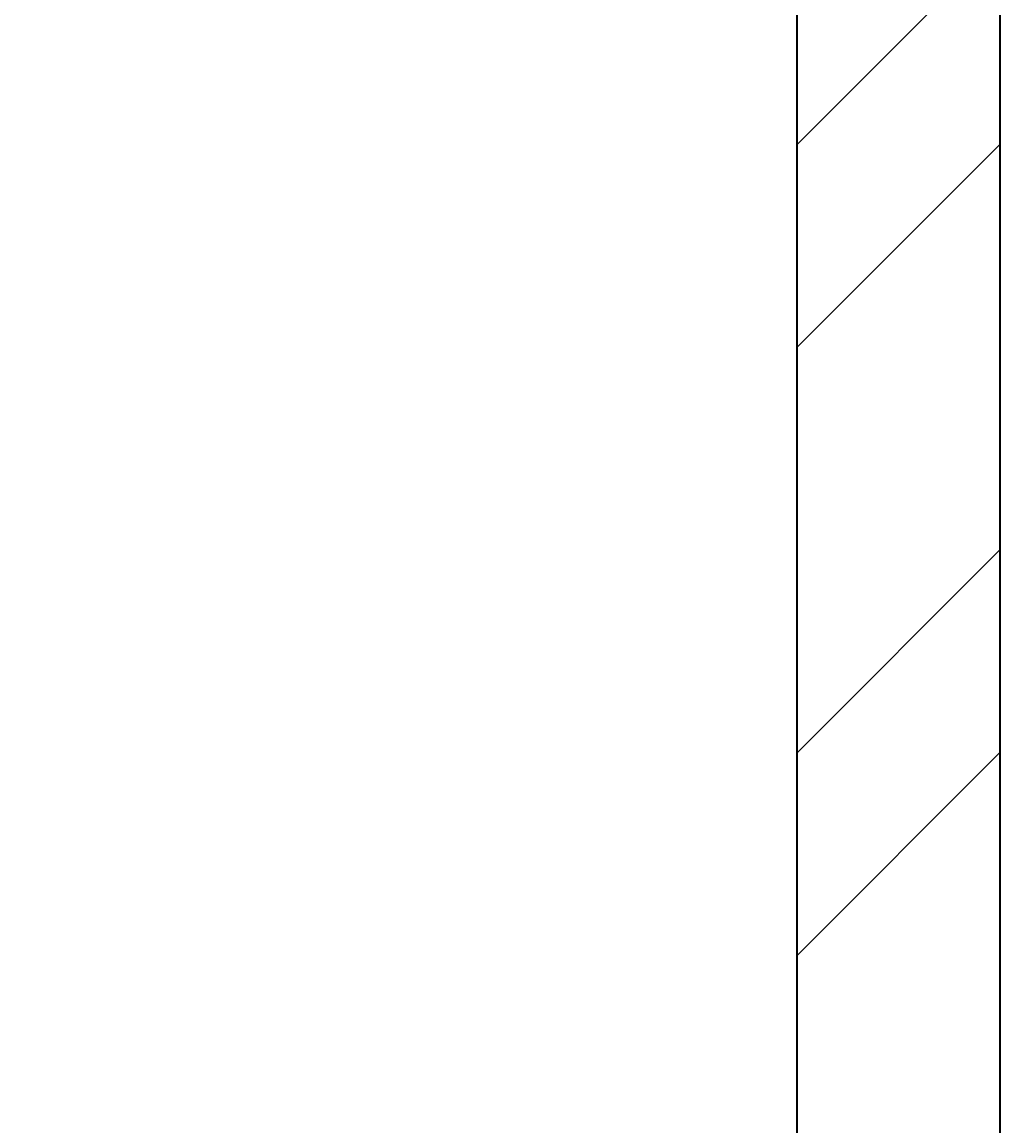
# Model space of a CAD drawing. Units: inches. Extents: x 1962 to 2771, y 1245 to 2660.
# Tile 79 of 114: x 2639 to 2661, y 2082 to 2107. Entities that reach past the tile are written whole.
import ezdxf

# ---------------------------------------------------------------- set-up
doc = ezdxf.new("R2010")
doc.units = ezdxf.units.IN
for name, color, linetype, lineweight in [('A-ANNO-DIMS', 2, 'Continuous', 18), ('A-WALL', 7, 'Continuous', 35), ('A-WALL-PATT', 252, 'Continuous', 13)]:
    doc.layers.add(name, color=color, linetype=linetype, lineweight=lineweight)
doc.styles.get("Standard").update_dxf_attribs({"font": 'arial.ttf'})
doc.dimstyles.get("Standard").update_dxf_attribs({"dimtxt": 0.18, "dimasz": 0.18, "dimexe": 0.18, "dimexo": 0.0625, "dimgap": 0.09, "dimtad": 0, "dimtih": 1, "dimtoh": 1, "dimdec": 4, "dimzin": 0, "dimdsep": 46, "dimtxsty": 'Standard', "dimcen": 0.09, "dimadec": 0, "dimazin": 0, "dimtfac": 1, "dimtdec": 4, "dimtofl": 0, "dimtmove": 0, "dimatfit": 3, "dimfxl": 1, "dimtolj": 1, "dimtzin": 0, "dimarcsym": 0})

# ---------------------------------------------------------------- blocks, each defined once
blk = doc.blocks.new('*D40')
at = {"layer": 'A-ANNO-DIMS', "color": 0, "lineweight": -2, "transparency": 16777216}
for p, q in [((2072.02, 2033.906), (2072.02, 2583.474)), ((2660.807, 2524.406), (2660.807, 2583.474)), ((2072.2, 2583.294), (2366.02, 2583.294)), ((2660.627, 2583.294), (2366.808, 2583.294))]:
    blk.add_line(p, q, dxfattribs=at)
at = {"layer": 'A-ANNO-DIMS', "color": 0, "transparency": 16777216}
for points in [[(2072.2, 2583.324), (2072.2, 2583.264), (2072.02, 2583.294)], [(2660.627, 2583.324), (2660.627, 2583.264), (2660.807, 2583.294)]]:
    blk.add_solid(points, dxfattribs=at)
at = {"layer": 'Defpoints', "color": 0, "transparency": 16777216}
for p in [(2660.807, 2583.294), (2660.807, 2524.344), (2072.02, 2033.844)]:
    blk.add_point(p, dxfattribs=at)
at = {"layer": 'A-ANNO-DIMS', "color": 0, "transparency": 16777216, "insert": (2366.414, 2583.294), "char_height": 0.18, "attachment_point": 5}
blk.add_mtext('\\A1;588.8', dxfattribs=at)

msp = doc.modelspace()

# ---------------------------------------------------------------- hatches: boundary and pattern name
at = {"layer": 'A-WALL-PATT'}
h = msp.add_hatch(dxfattribs=at)
h.set_pattern_fill('ANSI32', color=256)
h.paths.add_polyline_path([(2090.8074, 2467.3437), (2141.6481, 2467.3437), (2141.6481, 2469.5937), (2141.6481, 2471.8437), (2086.3074, 2471.8437), (2086.3074, 2422.5333), (2090.8074, 2422.5333)])
h.paths.add_polyline_path([(2282.7664, 2471.8437), (2204.8982, 2471.8437), (2204.8982, 2467.3437), (2234.8074, 2467.3437), (2234.8074, 2311.3437), (2228.7492, 2311.3437), (2228.7492, 2306.8437), (2234.8074, 2306.8437), (2331.9227, 2306.8437), (2331.9227, 2309.0937), (2331.9227, 2311.3437), (2239.3074, 2311.3437), (2239.3074, 2467.3437), (2282.7664, 2467.3437), (2282.7664, 2469.5937)])
h.paths.add_polyline_path([(2471.4531, 2519.8437), (2552.011, 2519.8437), (2564.3996, 2519.8437), (2564.3996, 2511.1389), (2568.8996, 2511.1389), (2568.8996, 2524.3437), (2466.9531, 2524.3437), (2466.9531, 2471.8437), (2450.0749, 2471.8437), (2446.4672, 2471.8437), (2446.4672, 2467.3437), (2450.0749, 2467.3437), (2475.9988, 2467.3437), (2475.9988, 2469.5937), (2475.9988, 2471.8437), (2471.4531, 2471.8437)])
h.paths.add_polyline_path([(2575.2231, 2469.5937), (2575.2231, 2471.8437), (2568.8996, 2471.8437), (2568.8996, 2487.1389), (2564.3996, 2487.1389), (2564.3996, 2471.8437), (2556.511, 2471.8437), (2499.2904, 2471.8437), (2499.2904, 2467.3437), (2507.8074, 2467.3437), (2507.8074, 2311.3437), (2414.863, 2311.3437), (2414.863, 2306.8437), (2512.3074, 2306.8437), (2517.0114, 2306.8437), (2517.0114, 2309.0937), (2517.0114, 2311.3437), (2512.3074, 2311.3437), (2512.3074, 2467.3437), (2575.2231, 2467.3437)])
h.paths.add_polyline_path([(2660.8074, 2471.8437), (2600.9602, 2471.8437), (2600.9602, 2467.3437), (2656.3074, 2467.3437), (2656.3074, 2432.5704), (2660.8074, 2432.5704)])
h.paths.add_polyline_path([(2660.8074, 2372.5704), (2656.3074, 2372.5704), (2656.3074, 2311.3437), (2600.276, 2311.3437), (2600.276, 2309.0937), (2600.276, 2306.8437), (2656.3074, 2306.8437), (2656.3074, 2296.2593), (2660.8074, 2296.2593)])
h.paths.add_polyline_path([(2572.3074, 2306.8437), (2577.1385, 2306.8437), (2577.1385, 2311.3437), (2551.082, 2311.3437), (2551.082, 2306.8437), (2567.8074, 2306.8437), (2567.8074, 2258.8437), (2540.0574, 2258.8437), (2540.0574, 2256.5937), (2540.0574, 2254.3437), (2567.8074, 2254.3437), (2656.3074, 2254.3437), (2656.3074, 2236.9085), (2660.8074, 2236.9085), (2660.8074, 2272.2593), (2656.3074, 2272.2593), (2656.3074, 2258.8437), (2572.3074, 2258.8437)])
h.paths.add_polyline_path([(2512.3074, 2254.3437), (2518.8716, 2254.3437), (2518.8716, 2256.5937), (2518.8716, 2258.8437), (2507.8074, 2258.8437), (2507.8074, 2177.8437), (2567.8074, 2177.8437), (2567.8074, 2172.9628), (2572.3074, 2172.9628), (2572.3074, 2177.8437), (2656.3074, 2177.8437), (2656.3074, 2166.4846), (2660.8074, 2166.4846), (2660.8074, 2200.9085), (2656.3074, 2200.9085), (2656.3074, 2182.3437), (2512.3074, 2182.3437)])
h.paths.add_polyline_path([(2656.3074, 2129.8437), (2572.3074, 2129.8437), (2572.3074, 2150.3044), (2570.0574, 2150.3044), (2567.8074, 2150.3044), (2567.8074, 2129.8437), (2507.8074, 2129.8437), (2507.8074, 2116.3027), (2510.0574, 2116.3027), (2512.3074, 2116.3027), (2512.3074, 2125.3437), (2567.8074, 2125.3437), (2572.3074, 2125.3437), (2656.3074, 2125.3437)])
h.paths.add_polyline_path([(2090.8074, 2362.5333), (2086.3074, 2362.5333), (2086.3074, 2298.6242), (2090.8074, 2298.6242), (2090.8074, 2306.8437), (2174.8074, 2306.8437), (2174.8074, 2286.4178), (2179.3074, 2286.4178), (2179.3074, 2306.8437), (2192.8641, 2306.8437), (2192.8641, 2309.0937), (2192.8641, 2311.3437), (2090.8074, 2311.3437)])
h.paths.add_polyline_path([(2209.156, 2258.8437), (2179.3074, 2258.8437), (2179.3074, 2263.2236), (2177.0574, 2263.2236), (2174.8074, 2263.2236), (2174.8074, 2258.8437), (2090.8074, 2258.8437), (2090.8074, 2274.6242), (2086.3074, 2274.6242), (2086.3074, 2238.2967), (2088.5574, 2238.2967), (2090.8074, 2238.2967), (2090.8074, 2254.3437), (2209.156, 2254.3437)])
h.paths.add_polyline_path([(2090.8074, 2177.8437), (2234.8074, 2177.8437), (2234.8074, 2173.1428), (2239.3074, 2173.1428), (2239.3074, 2258.8437), (2230.8442, 2258.8437), (2230.8442, 2256.5937), (2230.8442, 2254.3437), (2234.8074, 2254.3437), (2234.8074, 2182.3437), (2090.8074, 2182.3437), (2090.8074, 2202.2967), (2086.3074, 2202.2967), (2086.3074, 2140.0389), (2090.8074, 2140.0389)])
h.paths.add_polyline_path([(2090.8074, 2080.0389), (2086.3074, 2080.0389), (2086.3074, 2033.8437), (2090.8074, 2033.8437)], flags=17)
h.paths.add_polyline_path([(2244.9405, 2033.8437), (2239.3074, 2033.8437), (2239.3074, 2142.0665), (2237.2592, 2142.0665), (2234.8074, 2142.0665), (2234.8074, 2033.8437), (2090.8074, 2033.8437), (2076.5204, 2033.8437), (2072.0204, 2033.8437), (2072.0204, 2000.4493), (2076.5204, 2000.4493), (2076.5204, 2029.3437), (2090.8074, 2029.3437), (2244.9405, 2029.3437), (2244.9405, 2031.5937)])
h.paths.add_polyline_path([(2234.8074, 1933.3437), (2076.5204, 1933.3437), (2076.5204, 1952.4493), (2074.2704, 1952.4493), (2072.0204, 1952.4493), (2072.0204, 1933.3437), (2072.0204, 1928.8437), (2234.8074, 1928.8437)])
h.paths.add_polyline_path([(2090.8074, 1928.8437), (2086.3074, 1928.8437), (2086.3074, 1906.5013), (2090.8074, 1906.5013)])
h.paths.add_polyline_path([(2090.8074, 1846.5013), (2086.3074, 1846.5013), (2086.3074, 1769.9917), (2088.5574, 1769.9917), (2090.8074, 1769.9917), (2090.8074, 1780.3437), (2234.8074, 1780.3437), (2234.8074, 1708.3437), (2230.3764, 1708.3437), (2230.3764, 1703.8437), (2239.3074, 1703.8437), (2239.3074, 1792.6669), (2237.0574, 1792.6669), (2234.8074, 1792.6669), (2234.8074, 1784.8437), (2090.8074, 1784.8437)])
h.paths.add_polyline_path([(2239.3074, 1928.8437), (2244.9405, 1928.8437), (2244.9405, 1931.0937), (2244.9405, 1933.3437), (2234.8074, 1933.3437), (2234.8074, 1928.8437), (2234.8074, 1825.5949), (2239.3074, 1825.5949)])
h.paths.add_polyline_path([(2148.0425, 1649.0937), (2148.0425, 1651.3437), (2090.8074, 1651.3437), (2090.8074, 1646.8437), (2148.0425, 1646.8437)], flags=0)
h.paths.add_polyline_path([(2207.5601, 1708.3437), (2090.8074, 1708.3437), (2090.8074, 1703.8437), (2174.8074, 1703.8437), (2174.8074, 1651.3437), (2170.4457, 1651.3437), (2170.4457, 1646.8437), (2195.9924, 1646.8437), (2195.9924, 1649.0937), (2195.9924, 1651.3437), (2179.3074, 1651.3437), (2179.3074, 1703.8437), (2207.5601, 1703.8437), (2207.5601, 1706.0937)])
h.paths.add_polyline_path([(2090.8074, 1733.9917), (2086.3074, 1733.9917), (2086.3074, 1696.1032), (2088.5574, 1696.1032), (2090.8074, 1696.1032)])
h.paths.add_polyline_path([(2090.8074, 1672.1032), (2086.3074, 1672.1032), (2086.3074, 1600.3335), (2090.8074, 1600.3335)])
h.paths.add_polyline_path([(2090.8074, 1540.3335), (2086.3074, 1540.3335), (2086.3074, 1486.3437), (2139.6766, 1486.3437), (2139.6766, 1490.8437), (2090.8074, 1490.8437)])
h.paths.add_polyline_path([(2302.3876, 1490.8437), (2239.3074, 1490.8437), (2239.3074, 1646.8437), (2335.9994, 1646.8437), (2335.9994, 1651.3437), (2229.884, 1651.3437), (2229.884, 1646.8437), (2234.8074, 1646.8437), (2234.8074, 1490.8437), (2202.7103, 1490.8437), (2202.7103, 1488.5937), (2202.7103, 1486.3437), (2275.0699, 1486.3437), (2275.0699, 1475.772), (2279.5699, 1475.772), (2279.5699, 1486.3437), (2302.3876, 1486.3437)])
h.paths.add_polyline_path([(2279.5699, 1451.772), (2275.0699, 1451.772), (2275.0699, 1438.3437), (2174.8074, 1438.3437), (2174.8074, 1486.3437), (2179.7922, 1486.3437), (2179.7922, 1490.8437), (2163.3585, 1490.8437), (2163.3585, 1488.5937), (2163.3585, 1486.3437), (2170.3074, 1486.3437), (2170.3074, 1433.8437), (2279.5699, 1433.8437)])
h.paths.add_polyline_path([(2427.2363, 1490.8437), (2375.8074, 1490.8437), (2375.8074, 1646.8437), (2381.6401, 1646.8437), (2381.6401, 1651.3437), (2365.887, 1651.3437), (2365.887, 1649.0937), (2365.887, 1646.8437), (2371.3074, 1646.8437), (2371.3074, 1490.8437), (2327.5627, 1490.8437), (2327.5627, 1488.5937), (2327.5627, 1486.3437), (2371.3074, 1486.3437), (2371.3074, 1433.8437), (2375.8074, 1433.8437), (2375.8074, 1486.3437), (2427.2363, 1486.3437)])
h.paths.add_polyline_path([(2512.3074, 1646.8437), (2519.4351, 1646.8437), (2519.4351, 1649.0937), (2519.4351, 1651.3437), (2507.8074, 1651.3437), (2416.0063, 1651.3437), (2416.0063, 1649.0937), (2416.0063, 1646.8437), (2507.8074, 1646.8437), (2507.8074, 1490.8437), (2497.0532, 1490.8437), (2497.0532, 1488.5937), (2497.0532, 1486.3437), (2574.9344, 1486.3437), (2574.9344, 1476.0181), (2579.4344, 1476.0181), (2579.4344, 1486.3437), (2584.4872, 1486.3437), (2584.3074, 1490.8437), (2512.3074, 1490.8437)])
h.paths.add_polyline_path([(2470.5091, 1486.3437), (2473.9767, 1486.3437), (2473.9767, 1490.8437), (2449.6605, 1490.8437), (2449.6605, 1488.5937), (2449.6605, 1486.3437), (2466.0091, 1486.3437), (2466.0091, 1433.8437), (2470.5091, 1433.8437), (2579.4344, 1433.8437), (2579.4344, 1452.0181), (2574.9344, 1452.0181), (2574.9344, 1438.3437), (2554.5091, 1438.3437), (2470.5091, 1438.3437)])
h.paths.add_polyline_path([(2656.3074, 1490.8437), (2611.86, 1490.8437), (2611.86, 1486.3437), (2656.3074, 1486.3437)])
h.paths.add_polyline_path([(2660.8074, 1532.7007), (2658.5574, 1532.7007), (2656.3074, 1532.7007), (2656.3074, 1486.3437), (2660.8074, 1486.3437)])
h.paths.add_polyline_path([(2660.8074, 1664.9663), (2656.3074, 1664.9663), (2656.3074, 1651.3437), (2602.2313, 1651.3437), (2602.2313, 1646.8437), (2656.3074, 1646.8437), (2656.3074, 1592.7007), (2660.8074, 1592.7007)])
h.paths.add_polyline_path([(2660.8074, 1724.5221), (2656.3074, 1724.5221), (2656.3074, 1703.8437), (2542.4725, 1703.8437), (2542.4725, 1699.3437), (2567.8074, 1699.3437), (2567.8074, 1651.3437), (2552.7766, 1651.3437), (2552.7766, 1649.0937), (2552.7766, 1646.8437), (2577.2878, 1646.8437), (2577.2878, 1649.0937), (2577.2878, 1651.3437), (2572.3074, 1651.3437), (2572.3074, 1699.3437), (2656.3074, 1699.3437), (2656.3074, 1688.9663), (2660.8074, 1688.9663)])
h.paths.add_polyline_path([(2660.8074, 1880.6524), (2656.3074, 1880.6524), (2656.3074, 1832.8437), (2512.3074, 1832.8437), (2512.3074, 1837.8959), (2507.8074, 1837.8959), (2507.8074, 1828.3437), (2567.8074, 1828.3437), (2567.8074, 1804.3437), (2572.3074, 1804.3437), (2572.3074, 1828.3437), (2656.3074, 1828.3437), (2656.3074, 1818.6778), (2660.8074, 1818.6778)])
h.paths.add_polyline_path([(2660.8074, 1794.6778), (2656.3074, 1794.6778), (2656.3074, 1780.3437), (2572.3074, 1780.3437), (2572.3074, 1783.0303), (2570.0574, 1783.0303), (2567.8074, 1783.0303), (2567.8074, 1780.3437), (2507.8074, 1780.3437), (2507.8074, 1699.3437), (2517.8858, 1699.3437), (2517.8858, 1701.5937), (2517.8858, 1703.8437), (2512.3074, 1703.8437), (2512.3074, 1775.8437), (2656.3074, 1775.8437), (2656.3074, 1760.5221), (2660.8074, 1760.5221)])
h.paths.add_polyline_path([(2660.8074, 1981.3437), (2660.8074, 2020.2808), (2658.5574, 2020.2808), (2656.3074, 2020.2808), (2656.3074, 1981.3437), (2512.3074, 1981.3437), (2512.3074, 2086.6996), (2507.8074, 2086.6996), (2507.8074, 1981.3437), (2375.8074, 1981.3437), (2375.8074, 1986.8505), (2373.5574, 1986.8505), (2371.3074, 1986.8505), (2371.3074, 1973.2607), (2375.8074, 1973.2607), (2375.8074, 1976.8437), (2507.8074, 1976.8437), (2507.8074, 1865.4281), (2510.0574, 1865.4281), (2512.3074, 1865.4281), (2512.3074, 1976.8437), (2660.8074, 1976.8437)])
h.paths.add_polyline_path([(2375.8074, 1940.297), (2373.5574, 1940.297), (2371.3074, 1940.297), (2371.3074, 1933.3437), (2278.4434, 1933.3437), (2278.4434, 1928.8437), (2371.3074, 1928.8437), (2371.3074, 1651.3437), (2375.8074, 1651.3437)])
h.paths.add_polyline_path([(2660.8074, 1976.8437), (2656.3074, 1976.8437), (2656.3074, 1940.6524), (2660.8074, 1940.6524)], flags=17)
h.paths.add_polyline_path([(2660.8074, 2142.4846), (2656.3074, 2142.4846), (2656.3074, 2080.2808), (2660.8074, 2080.2808)])
h.paths.add_polyline_path([(2381.4189, 2311.3437), (2375.8074, 2311.3437), (2375.8074, 2467.3437), (2424.7242, 2467.3437), (2424.7242, 2469.5937), (2424.7242, 2471.8437), (2375.8074, 2471.8437), (2375.8074, 2524.3437), (2371.3074, 2524.3437), (2371.3074, 2471.8437), (2307.2097, 2471.8437), (2307.2097, 2467.3437), (2371.3074, 2467.3437), (2371.3074, 2311.3437), (2366.8901, 2311.3437), (2366.8901, 2306.8437), (2371.3074, 2306.8437), (2371.3074, 2033.8437), (2279.6589, 2033.8437), (2279.6589, 2029.3437), (2371.3074, 2029.3437), (2371.3074, 2014.2598), (2375.8074, 2014.2598), (2375.8074, 2306.8437), (2381.4189, 2306.8437)])
h.paths.add_polyline_path([(2263.3074, 2524.3437), (2170.3074, 2524.3437), (2170.3074, 2519.8437), (2170.3074, 2471.8437), (2165.0312, 2471.8437), (2165.0312, 2467.3437), (2179.6721, 2467.3437), (2179.6721, 2469.5161), (2179.6721, 2471.8437), (2174.8074, 2471.8437), (2174.8074, 2519.8437), (2258.8074, 2519.8437), (2258.8074, 2511.6436), (2263.3074, 2511.6436)])
h.paths.add_polyline_path([(2245.0232, 1361.4123), (2492.9468, 1361.4123), (2492.9468, 1398.505), (2245.0232, 1398.505)], flags=9)
h.paths.add_polyline_path([(2388.1434, 2086.6936), (2425.0704, 2086.6936), (2425.0704, 2105.3509), (2388.1434, 2105.3509)], flags=9)
h.paths.add_polyline_path([(2404.922, 2242.6744), (2445.7337, 2242.6744), (2445.7337, 2261.3318), (2404.922, 2261.3318)], flags=9)
h.paths.add_polyline_path([(2269.4107, 2156.7935), (2306.3378, 2156.7935), (2306.3378, 2175.4508), (2269.4107, 2175.4508)], flags=9)
h.paths.add_polyline_path([(2269.3277, 2233.4343), (2306.2547, 2233.4343), (2306.2547, 2252.0917), (2269.3277, 2252.0917)], flags=9)
h.paths.add_polyline_path([(2431.6052, 2320.6922), (2470.4456, 2320.6922), (2470.4456, 2339.3495), (2431.6052, 2339.3495)], flags=25)
h.paths.add_polyline_path([(2249.6902, 2315.7608), (2288.5306, 2315.7608), (2288.5306, 2334.4182), (2249.6902, 2334.4182)], flags=25)
h.paths.add_polyline_path([(2096.9301, 2314.3181), (2135.7704, 2314.3181), (2135.7704, 2332.9755), (2096.9301, 2332.9755)], flags=25)
h.paths.add_polyline_path([(2134.3475, 2285.7089), (2161.4655, 2285.7089), (2161.4655, 2304.3662), (2134.3475, 2304.3662)], flags=9)
h.paths.add_polyline_path([(2126.5155, 2209.4076), (2159.9227, 2209.4076), (2159.9227, 2228.065), (2126.5155, 2228.065)], flags=25)
h.paths.add_polyline_path([(2110.5753, 2141.5299), (2149.4157, 2141.5299), (2149.4157, 2160.1872), (2110.5753, 2160.1872)], flags=25)
h.paths.add_polyline_path([(2249.8618, 1968.3317), (2286.3966, 1968.3317), (2286.3966, 1986.989), (2249.8618, 1986.989)], flags=9)
h.paths.add_polyline_path([(2395.9507, 1777.0051), (2436.7624, 1777.0051), (2436.7624, 1795.6625), (2395.9507, 1795.6625)], flags=9)
h.paths.add_polyline_path([(2398.5259, 1888.5651), (2435.0062, 1888.5651), (2435.0062, 1907.2224), (2398.5259, 1907.2224)], flags=25)
h.paths.add_polyline_path([(2259.3506, 1728.3559), (2296.2776, 1728.3559), (2296.2776, 1747.0132), (2259.3506, 1747.0132)], flags=9)
h.paths.add_polyline_path([(2271.3698, 1845.268), (2308.2968, 1845.268), (2308.2968, 1863.9253), (2271.3698, 1863.9253)], flags=9)
h.paths.add_polyline_path([(2120.9355, 1786.3027), (2159.7759, 1786.3027), (2159.7759, 1804.9601), (2120.9355, 1804.9601)], flags=25)
h.paths.add_polyline_path([(2121.3164, 1732.1043), (2154.7236, 1732.1043), (2154.7236, 1750.7616), (2121.3164, 1750.7616)], flags=25)
h.paths.add_polyline_path([(2118.3706, 1678.8997), (2147.5282, 1678.8997), (2147.5282, 1697.557), (2118.3706, 1697.557)], flags=25)
h.paths.add_polyline_path([(2385.9227, 1493.557), (2424.763, 1493.557), (2424.763, 1512.2143), (2385.9227, 1512.2143)], flags=25)
h.paths.add_polyline_path([(2248.7058, 1500.0256), (2287.5462, 1500.0256), (2287.5462, 1518.6829), (2248.7058, 1518.6829)], flags=25)
h.paths.add_polyline_path([(2104.1669, 1617.3771), (2143.0073, 1617.3771), (2143.0073, 1636.0344), (2104.1669, 1636.0344)], flags=9)
h.paths.add_polyline_path([(2096.0714, 1447.8824), (2137.3845, 1447.8824), (2137.3845, 1458.1859), (2096.0714, 1458.1859)], flags=9)
h.paths.add_polyline_path([(2180.6114, 1440.325), (2209.7689, 1440.325), (2209.7689, 1458.9823), (2180.6114, 1458.9823)], flags=25)
h.paths.add_polyline_path([(2316.1698, 1447.9637), (2357.4829, 1447.9637), (2357.4829, 1458.2673), (2316.1698, 1458.2673)], flags=9)
h.paths.add_polyline_path([(2397.6187, 1447.9637), (2438.9318, 1447.9637), (2438.9318, 1458.2673), (2397.6187, 1458.2673)], flags=9)
h.paths.add_polyline_path([(2473.0778, 1439.5953), (2502.2354, 1439.5953), (2502.2354, 1458.2527), (2473.0778, 1458.2527)], flags=25)
h.paths.add_polyline_path([(2589.7027, 1447.8819), (2631.0158, 1447.8819), (2631.0158, 1458.1855), (2589.7027, 1458.1855)], flags=9)
h.paths.add_polyline_path([(2522.4009, 1497.5285), (2561.2413, 1497.5285), (2561.2413, 1516.1859), (2522.4009, 1516.1859)], flags=25)
h.paths.add_polyline_path([(2579.6565, 1671.3482), (2608.8141, 1671.3482), (2608.8141, 1690.0056), (2579.6565, 1690.0056)], flags=25)
h.paths.add_polyline_path([(2544.7038, 1725.5064), (2578.1111, 1725.5064), (2578.1111, 1744.1637), (2544.7038, 1744.1637)], flags=25)
h.paths.add_polyline_path([(2578.1191, 1807.472), (2607.2766, 1807.472), (2607.2766, 1826.1293), (2578.1191, 1826.1293)], flags=25)
h.paths.add_polyline_path([(2595.0614, 1835.1839), (2633.9018, 1835.1839), (2633.9018, 1853.8413), (2595.0614, 1853.8413)], flags=25)
h.paths.add_polyline_path([(2567.0097, 2097.7035), (2605.8501, 2097.7035), (2605.8501, 2116.3609), (2567.0097, 2116.3609)], flags=9)
h.paths.add_polyline_path([(2586.644, 2134.6454), (2615.8015, 2134.6454), (2615.8015, 2153.3027), (2586.644, 2153.3027)], flags=9)
h.paths.add_polyline_path([(2544.6185, 2212.6783), (2578.0258, 2212.6783), (2578.0258, 2231.3356), (2544.6185, 2231.3356)], flags=25)
h.paths.add_polyline_path([(2577.0273, 2256.9023), (2606.1849, 2256.9023), (2606.1849, 2275.5597), (2577.0273, 2275.5597)], flags=24)
h.paths.add_polyline_path([(2605.2683, 2315.2821), (2644.1087, 2315.2821), (2644.1087, 2333.9395), (2605.2683, 2333.9395)], flags=25)
h.paths.add_polyline_path([(2583.1244, 2496.1815), (2624.4375, 2496.1815), (2624.4375, 2506.4851), (2583.1244, 2506.4851)], flags=9)
h.paths.add_polyline_path([(2474.761, 2497.0823), (2503.9185, 2497.0823), (2503.9185, 2515.7397), (2474.761, 2515.7397)], flags=25)
h.paths.add_polyline_path([(2387.5787, 2494.2563), (2428.902, 2494.2563), (2428.902, 2504.5598), (2387.5787, 2504.5598)], flags=9)
h.paths.add_polyline_path([(2300.1657, 2500.1564), (2341.4788, 2500.1564), (2341.4788, 2510.46), (2300.1657, 2510.46)], flags=25)
h.paths.add_polyline_path([(2176.8589, 2497.5843), (2206.0165, 2497.5843), (2206.0165, 2516.2416), (2176.8589, 2516.2416)], flags=25)
h.paths.add_polyline_path([(2097.4668, 2494.9762), (2138.7799, 2494.9762), (2138.7799, 2505.2798), (2097.4668, 2505.2798)], flags=9)

# ---------------------------------------------------------------- linework, layer by layer
at = {"layer": 'A-WALL'}
for p, q in [((2660.8074, 2471.8437), (2660.8074, 1976.8437)), ((2656.3074, 2177.8437), (2656.3074, 1981.3437))]:
    msp.add_line(p, q, dxfattribs=at)

# ---------------------------------------------------------------- dimensions: what is measured, and where the dimension line sits
at = {"layer": 'A-ANNO-DIMS'}
dim = msp.add_linear_dim(base=(2660.8074, 2583.2937), p1=(2072.0204, 2033.8437), p2=(2660.8074, 2524.3437), dimstyle='Standard', override={"dimdec": 1, "dimlfac": 1, "dimrnd": 0, "dimzin": 0, "dimdsep": 46, "dimlunit": 2}, dxfattribs=at)
dim.commit()
dim.dimension.update_dxf_attribs({"geometry": '*D40', "text_midpoint": (2366.4139, 2583.2937)})

doc.saveas('drawing.dxf')
